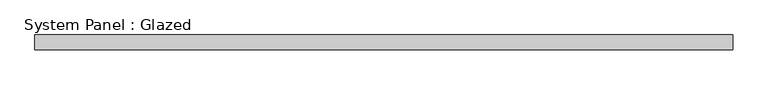
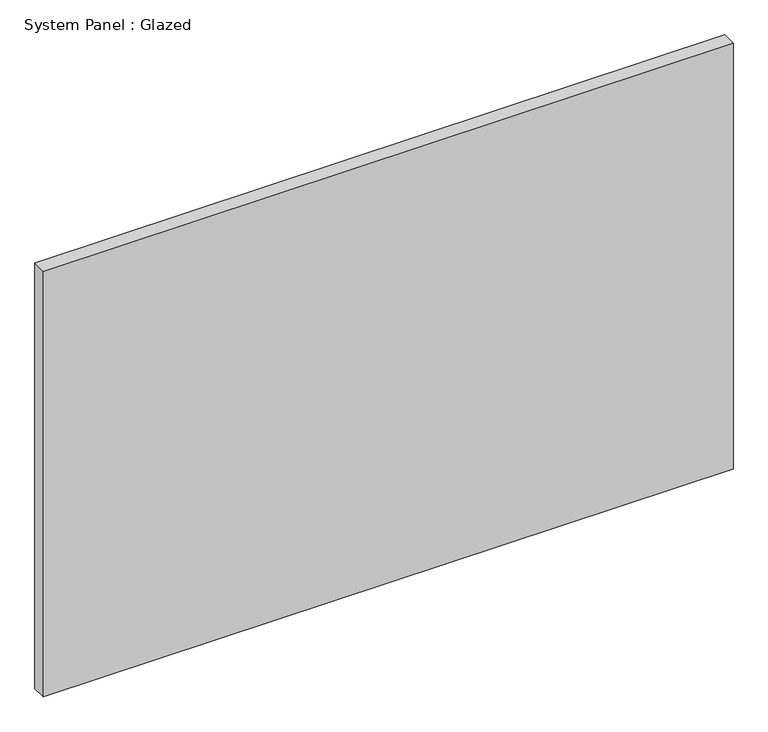
"""IFC4 building model written with IfcOpenShell, lengths in millimetres: plate geometry, System Panel : Glazed."""

from ifc_helpers import new_model, si_unit, origin, origin_with_axes, place, context, project, spatial, polyline, outline, extrude, source, transform, mapped, element, save


def system_panel_glazed_876b4d55(model_context):
    return source(origin(), model_context, "Body", "SweptSolid", [
        extrude(outline(polyline([(603.2499999, 19.05), (-603.2499999, 19.05), (-603.2499999, 44.45), (603.2499999, 44.45), (603.2499999, 19.05)])), origin_with_axes(), (0.0, 0.0, 1.0), 787.4),
    ])


if __name__ == "__main__":
    model = new_model("IFC4")
    model_context = context("Model", 3, world=origin())
    ifc_project = project(units=[si_unit("LENGTHUNIT", "METRE", prefix="MILLI")], contexts=[model_context])
    site = spatial("IfcSite", under=ifc_project)
    building = spatial("IfcBuilding", under=site)
    placement = place(None, origin())
    system_panel_glazed_shape = system_panel_glazed_876b4d55(model_context)
    element("IfcPlate", 1, ObjectType="System Panel : Glazed", at=placement, inside=building, context=model_context, shape_type="MappedRepresentation", body=[
        mapped(system_panel_glazed_shape, transform((0.0, 0.0, 0.0), x_axis=(1.0, 0.0, 0.0), y_axis=(0.0, 1.0, 0.0), z_axis=(0.0, 0.0, 1.0))),
    ])
    save(model, "model.ifc")

# Revit data of these elements
# Type "System Panel : Glazed"
#   Construction Type Id = "GSP4R"
#   Analytic Construction = "1/8 in Pilkington single glazing"
#   Visual Light Transmittance = 0.9
#   Solar Heat Gain Coefficient = 0.86
#   Heat Transfer Coefficient (U) = 1.18115 BTU/(h·ft²·°F)
#   Define Thermal Properties by = 1
# Element 1 (IfcPlate, "System Panel : Glazed")
#   Materials on its faces: "Glass"
# Materials
#   "Glass": class "Glass", colour RGB 0 128 192, transparency 0.75, Description = "Soda Lime Glass", Cost = 0
